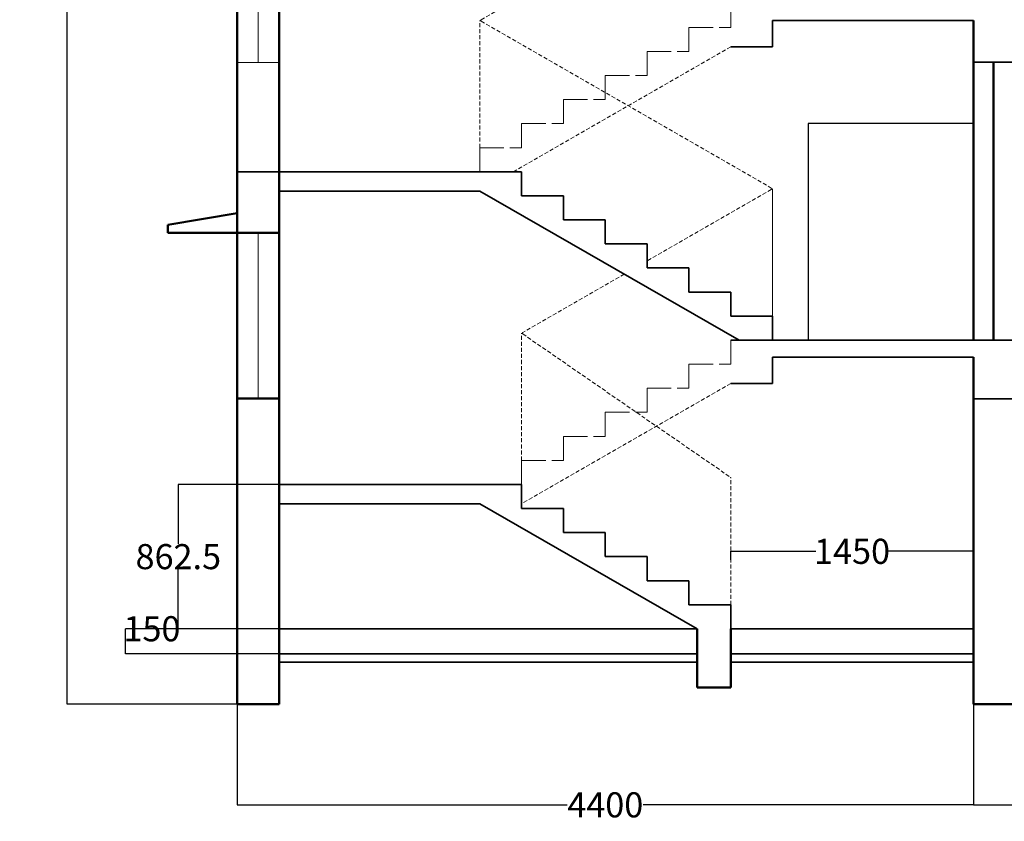
# Model space of a CAD drawing. Units: millimetres. Extents: x -1193 to 12449, y -949 to 12489.
# Tile 1 of 2: x -1193 to 4692, y -949 to 3842. Entities that reach past the tile are written whole.
import ezdxf

# ---------------------------------------------------------------- set-up
doc = ezdxf.new("R2010")
doc.units = ezdxf.units.MM
doc.header["$LTSCALE"] = 12
doc.header["$MEASUREMENT"] = 0
doc.linetypes.add('ACAD_ISO02W100', pattern=[15, 12, -3])
doc.linetypes.add('HIDDEN', pattern=[0.375, 0.25, -0.125])
for name, color, linetype, lineweight in [('A-ANNO-DIMS', 2, 'Continuous', 18), ('A-DOOR', 3, 'Continuous', 25), ('A-FLOR', 7, 'Continuous', 35), ('A-FLOR-HRAL-BYND', 8, 'ACAD_ISO02W100', 18), ('A-FLOR-HRAL-HIDN', 8, 'HIDDEN', 18), ('A-FLOR-STRS', 7, 'Continuous', 35), ('A-FLOR-STRS-BYND', 8, 'ACAD_ISO02W100', 18), ('A-FLOR-STRS-HIDN', 8, 'HIDDEN', 18), ('A-GLAZ', 4, 'Continuous', 18), ('A-WALL', 7, 'Continuous', 50), ('A-WALL-BYND', 8, 'ACAD_ISO02W100', 18), ('S-BEAM', 1, 'Continuous', 35), ('S-COLS', 1, 'Continuous', 50), ('S-FNDN', 1, 'Continuous', 50)]:
    doc.layers.add(name, color=color, linetype=linetype, lineweight=lineweight)
doc.styles.get("Standard").update_dxf_attribs({"font": 'arial.ttf'})
doc.dimstyles.get("Standard").update_dxf_attribs({"dimtxt": 150, "dimasz": 0.18, "dimexe": 0.18, "dimexo": 0.0625, "dimgap": 0.09, "dimtad": 0, "dimtih": 1, "dimtoh": 1, "dimdec": 0, "dimzin": 0, "dimdsep": 46, "dimtxsty": 'Standard', "dimcen": 0.09, "dimadec": 0, "dimazin": 0, "dimtfac": 1, "dimtdec": 0, "dimtofl": 0, "dimtmove": 0, "dimatfit": 3, "dimfxl": 1, "dimtolj": 1, "dimtzin": 0, "dimarcsym": 0})

# ---------------------------------------------------------------- blocks, each defined once
blk = doc.blocks.new('*D3')
at = {"layer": 'A-ANNO-DIMS', "color": 0, "lineweight": -2, "ltscale": 8, "transparency": 16777216}
for p, q in [((3057.011297115449, 613.4543490366777), (3057.011297115449, 664.80195058669)), ((3057.191297115449, 664.6219505866902), (3565.260314850783, 664.6219505866902)), ((4506.831297115448, 664.6219505866902), (3998.762279380115, 664.6219505866902)), ((4507.011297115449, 613.4543490366777), (4507.011297115449, 664.80195058669))]:
    blk.add_line(p, q, dxfattribs=at)
at = {"layer": 'A-ANNO-DIMS', "color": 0, "ltscale": 8, "transparency": 16777216}
for points in [[(3057.191297115449, 664.6519505866901), (3057.191297115449, 664.5919505866902), (3057.011297115449, 664.6219505866902)], [(4506.831297115448, 664.6519505866901), (4506.831297115448, 664.5919505866902), (4507.011297115449, 664.6219505866902)]]:
    blk.add_solid(points, dxfattribs=at)
at = {"layer": 'Defpoints', "color": 0, "ltscale": 8, "transparency": 16777216}
for p in [(4507.011297115449, 664.6219505866902), (3057.011297115449, 613.3918490366777), (4507.011297115449, 613.3918490366777)]:
    blk.add_point(p, dxfattribs=at)
at = {"layer": 'A-ANNO-DIMS', "color": 0, "ltscale": 8, "transparency": 16777216, "insert": (3782.011297115449, 664.6219505866902), "char_height": 150, "attachment_point": 5}
blk.add_mtext('\\A1;1450', dxfattribs=at)
blk = doc.blocks.new('*D5')
at = {"layer": 'A-ANNO-DIMS', "color": 0, "lineweight": -2, "ltscale": 8, "transparency": 16777216}
for p, q in [((356.9487971154486, 201.7493925244232), (-561.4085524250191, 201.749392524423)), ((-561.2285524250191, 201.749392524423), (-561.2285524250191, 201.929392524423)), ((-561.2285524250191, 201.929392524423), (-561.0485524250192, 201.929392524423)), ((-561.2285524250191, 51.92939252442293), (-561.2285524250191, 201.569392524423)), ((356.9487971154487, 51.74939252442309), (-561.4085524250191, 51.74939252442293))]:
    blk.add_line(p, q, dxfattribs=at)
at = {"layer": 'A-ANNO-DIMS', "color": 0, "ltscale": 8, "transparency": 16777216}
for points in [[(-561.258552425019, 201.569392524423), (-561.1985524250192, 201.569392524423), (-561.2285524250191, 201.749392524423)], [(-561.258552425019, 51.92939252442293), (-561.1985524250192, 51.92939252442293), (-561.2285524250191, 51.74939252442293)]]:
    blk.add_solid(points, dxfattribs=at)
at = {"layer": 'Defpoints', "color": 0, "ltscale": 8, "transparency": 16777216}
for p in [(-561.2285524250191, 201.749392524423), (357.0112971154486, 201.7493925244232), (357.0112971154487, 51.74939252442309)]:
    blk.add_point(p, dxfattribs=at)
at = {"layer": 'A-ANNO-DIMS', "color": 0, "ltscale": 8, "transparency": 16777216, "insert": (-402.5683750716766, 201.9293925244231), "char_height": 150, "attachment_point": 5}
blk.add_mtext('\\A1;150', dxfattribs=at)
blk = doc.blocks.new('STAIR-FLIGHT-LANDING-TYP')
at = {"ltscale": 8}
for p, q in [((1200, 1006.25), (-5.68e-14, 1006.25)), ((1200, 890.8972800494066), (-5.68e-14, 890.8972800494066))]:
    blk.add_line(p, q, dxfattribs=at)
for p, q in [((1450, 1006.25), (1200, 1006.25)), ((1450, 862.5), (1450, 1006.25)), ((1700, 862.5), (1450, 862.5)), ((1700, 718.75), (1700, 862.5)), ((1950, 718.75), (1700, 718.75)), ((1950, 575), (1950, 718.75)), ((2200, 575), (1950, 575)), ((2200, 431.25), (2200, 575)), ((2450, 431.25), (2200, 431.25)), ((2450, 287.5), (2450, 431.25)), ((2700, 287.5), (2450, 287.5)), ((2700, 143.75), (2700, 287.5)), ((2950, 143.75), (2700, 143.75)), ((2950, 0), (2950, 143.75))]:
    blk.add_line(p, q)
blk.add_lwpolyline([(1200, 890.8972800494066), (2749.386573998968, 0)], dxfattribs=at)
blk = doc.blocks.new('STAIR-RETURN-TYP')
for p, q in [((1500, 862.5), (1500, 1006.25)), ((1500, 1006.25), (1750, 1006.25)), ((1250, 718.75), (1250, 862.5)), ((1250, 862.5), (1500, 862.5)), ((999.9999999999995, 575), (999.9999999999995, 718.75)), ((999.9999999999995, 718.75), (1250, 718.75)), ((749.9999999999995, 431.25), (749.9999999999995, 575)), ((749.9999999999995, 575), (999.9999999999995, 575)), ((499.9999999999995, 287.5), (499.9999999999995, 431.25)), ((499.9999999999995, 431.25), (749.9999999999995, 431.25)), ((249.9999999999996, 143.75), (249.9999999999996, 287.5)), ((249.9999999999996, 287.5), (499.9999999999995, 287.5)), ((-4.547e-13, 0), (-4.547e-13, 143.75)), ((-4.547e-13, 143.75), (249.9999999999996, 143.75))]:
    blk.add_line(p, q)
blk = doc.blocks.new('DOOR-STAIR-OPENING')
at = {"ltscale": 8}
for p, q in [((988.0075403151895, 1293.961950984857), (0, 1293.961950984857)), ((0, 1293.961950984857), (0, 0))]:
    blk.add_line(p, q, dxfattribs=at)
blk = doc.blocks.new('BEAM-DROP-250x250')
for p, q in [((0, 250), (0, 0)), ((250, 0), (250, 250)), ((0, 0), (250, 0))]:
    blk.add_line(p, q)
blk = doc.blocks.new('*D28')
at = {"layer": 'A-ANNO-DIMS', "color": 0, "lineweight": -2, "ltscale": 8, "transparency": 16777216}
for p, q in [((106.948797, 11788.48548), (-909.1941130000021, 11788.48548)), ((-909.0141130000022, 11788.30548), (-909.0141130000007, 5846.844544276263)), ((-909.0141129999995, -248.0706070000003), (-909.0141130000007, 5693.39032872374)), ((106.948797, -248.2506070000001), (-909.1941129999994, -248.2506070000003))]:
    blk.add_line(p, q, dxfattribs=at)
at = {"layer": 'A-ANNO-DIMS', "color": 0, "ltscale": 8, "transparency": 16777216}
for points in [[(-909.0441130000021, 11788.30548), (-908.9841130000023, 11788.30548), (-909.0141130000022, 11788.48548)], [(-909.0441129999996, -248.0706070000003), (-908.9841129999996, -248.0706070000003), (-909.0141129999995, -248.2506070000003)]]:
    blk.add_solid(points, dxfattribs=at)
at = {"layer": 'Defpoints', "color": 0, "ltscale": 8, "transparency": 16777216}
for p in [(-909.0141130000022, 11788.48548), (107.011297, 11788.48548), (107.011297, -248.2506070000001)]:
    blk.add_point(p, dxfattribs=at)
at = {"layer": 'A-ANNO-DIMS', "color": 0, "ltscale": 8, "transparency": 16777216, "insert": (-909.014112999999, 5770.117436500001), "char_height": 150, "attachment_point": 5}
blk.add_mtext('\\A1;12037', dxfattribs=at)
blk = doc.blocks.new('*D29')
at = {"layer": 'A-ANNO-DIMS', "color": 0, "lineweight": -2, "ltscale": 8, "transparency": 16777216}
for p, q in [((107.011297, -248.313107), (107.0112969999999, -850.430607)), ((4507.011297, -248.313107), (4507.011297, -850.430607)), ((107.1912969999999, -850.250607), (2080.181869987722, -850.250607)), ((4506.831297, -850.250607), (2533.840724012279, -850.250607))]:
    blk.add_line(p, q, dxfattribs=at)
at = {"layer": 'A-ANNO-DIMS', "color": 0, "ltscale": 8, "transparency": 16777216}
for points in [[(107.1912969999999, -850.2206069999999), (107.1912969999999, -850.280607), (107.0112969999999, -850.250607)], [(4506.831297, -850.2206069999999), (4506.831297, -850.280607), (4507.011297, -850.250607)]]:
    blk.add_solid(points, dxfattribs=at)
at = {"layer": 'Defpoints', "color": 0, "ltscale": 8, "transparency": 16777216}
for p in [(107.011297, -248.250607), (4507.011297, -248.250607), (4507.011297, -850.250607)]:
    blk.add_point(p, dxfattribs=at)
at = {"layer": 'A-ANNO-DIMS', "color": 0, "ltscale": 8, "transparency": 16777216, "insert": (2307.011297, -850.250607), "char_height": 150, "attachment_point": 5}
blk.add_mtext('\\A1;4400', dxfattribs=at)
blk = doc.blocks.new('*D30')
at = {"layer": 'A-ANNO-DIMS', "color": 0, "lineweight": -2, "ltscale": 8, "transparency": 16777216}
for p, q in [((5559.096303, 2520.911284), (5559.096303, -850.4306069999998)), ((4507.011297, -248.313107), (4507.011297, -850.430607)), ((4507.191297000001, -850.250607), (4816.814413915416, -850.250607)), ((5558.916303, -850.250607), (5249.293186084583, -850.250607))]:
    blk.add_line(p, q, dxfattribs=at)
at = {"layer": 'A-ANNO-DIMS', "color": 0, "ltscale": 8, "transparency": 16777216}
for points in [[(4507.191297000001, -850.2206069999999), (4507.191297000001, -850.280607), (4507.011297, -850.250607)], [(5558.916303, -850.2206069999999), (5558.916303, -850.280607), (5559.096303, -850.250607)]]:
    blk.add_solid(points, dxfattribs=at)
at = {"layer": 'Defpoints', "color": 0, "ltscale": 8, "transparency": 16777216}
for p in [(5559.096303, 2520.973784), (4507.011297, -248.250607), (5559.096303, -850.250607)]:
    blk.add_point(p, dxfattribs=at)
at = {"layer": 'A-ANNO-DIMS', "color": 0, "ltscale": 8, "transparency": 16777216, "insert": (5033.0538, -850.250607), "char_height": 150, "attachment_point": 5}
blk.add_mtext('\\A1;1052', dxfattribs=at)
blk = doc.blocks.new('*D49')
at = {"layer": 'A-ANNO-DIMS', "color": 0, "lineweight": -2, "ltscale": 8, "transparency": 16777216}
for p, q in [((356.9487970000001, 1064.249393), (-245.1687030000003, 1064.249393)), ((-244.9887030000003, 1064.069393), (-244.9887030000002, 709.6753411582539)), ((-244.9887030000001, 201.929393), (-244.9887030000002, 556.3234448417464)), ((356.9487970000001, 201.7493930000001), (-245.168703, 201.749393))]:
    blk.add_line(p, q, dxfattribs=at)
at = {"layer": 'A-ANNO-DIMS', "color": 0, "ltscale": 8, "transparency": 16777216}
for points in [[(-245.0187030000003, 1064.069393), (-244.9587030000003, 1064.069393), (-244.9887030000003, 1064.249393)], [(-245.0187030000001, 201.929393), (-244.9587030000001, 201.929393), (-244.9887030000001, 201.749393)]]:
    blk.add_solid(points, dxfattribs=at)
at = {"layer": 'Defpoints', "color": 0, "ltscale": 8, "transparency": 16777216}
for p in [(-244.9887030000003, 1064.249393), (357.0112970000001, 1064.249393), (357.0112970000001, 201.7493930000001)]:
    blk.add_point(p, dxfattribs=at)
at = {"layer": 'A-ANNO-DIMS', "color": 0, "ltscale": 8, "transparency": 16777216, "insert": (-244.988703, 632.999393), "char_height": 150, "attachment_point": 5}
blk.add_mtext('\\A1;862.5', dxfattribs=at)

msp = doc.modelspace()

# ---------------------------------------------------------------- linework, layer by layer
at = {"layer": 'A-FLOR', "ltscale": 8}
for p, q in [((3307.011297115448, 3837.249392524423), (4507.011297115449, 3837.249392524423)), ((3057.011297115449, 1926.749392524423), (4507.011297115449, 1926.749392524423))]:
    msp.add_line(p, q, dxfattribs=at)
at = {"layer": 'A-FLOR'}
for p, q in [((4507.011297115449, 1926.749392524423), (10755.12605663696, 1926.749392524423)), ((3307.011297115448, 1825.149392524423), (4507.011297115449, 1825.149392524423)), ((357.0112971154486, 201.749392524423), (2856.397871114416, 201.749392524423)), ((3057.011297115449, 201.749392524423), (4507.011297115449, 201.749392524423)), ((357.0112971154486, 51.74939252442306), (2856.397871114416, 51.74939252442306)), ((357.0112971154486, 1.749392524423061), (2856.397871114416, 1.749392524423061)), ((3057.011297115448, 51.74939252442306), (4507.011297115449, 51.74939252442306)), ((3057.011297115448, 1.749392524423061), (4507.011297115449, 1.749392524423061))]:
    msp.add_line(p, q, dxfattribs=at)
at = {"layer": 'A-FLOR-HRAL-BYND', "ltscale": 8}
msp.add_line((3307.011297115449, 2070.499392524423), (3307.011297115449, 2830.999392524419), dxfattribs=at)
at = {"layer": 'A-FLOR-HRAL-HIDN', "ltscale": 8}
for p, q in [((1564.54961279421, 3841.583924039707), (2420.40023628885, 4333.698032549124)), ((1557.011297115449, 3076.749392524423), (1557.011297115449, 3837.249392524419)), ((1564.54961279421, 3832.914861009131), (3299.472981436688, 2835.333924039707)), ((3299.472981436688, 2826.664861009131), (2557.011297115449, 2399.749392524419)), ((2420.400236288849, 2321.198032549124), (1813.880505755374, 1972.449187492376)), ((1807.011297115449, 1207.999392524423), (1807.011297115449, 1968.499392524419)), ((1813.533234977974, 1963.999255399276), (3054.850923514139, 1107.490050309322)), ((3057.011297115449, 345.499392524423), (3057.011297115449, 1103.37464973151))]:
    msp.add_line(p, q, dxfattribs=at)
for centre, start, end in [((1567.0419684155, 3837.249392524419), 119.8989018386145, 240.1010981613854), ((3296.980625815397, 2830.999392524419), 299.8989018386146, 60.10109816138544), ((1816.372861376665, 1968.114655977089), 119.8989018386145, 235.3943244483614), ((3052.011297115449, 1103.37464973151), 0, 55.39432444836143)]:
    msp.add_arc(centre, 5, start, end, dxfattribs=at)
at = {"layer": 'A-FLOR-STRS', "ltscale": 8}
for p, q in [((3307.011297115449, 3679.746672573831), (3307.011297115448, 3837.249392524423)), ((3057.011297115449, 3679.746672573831), (3307.011297115449, 3679.746672573831)), ((357.0112971154486, 2932.999392524423), (107.0112971154485, 2932.999392524423)), ((3307.011297115449, 1667.64667257383), (3307.011297115448, 1825.149392524423)), ((3057.011297115449, 1667.64667257383), (3307.011297115449, 1667.64667257383))]:
    msp.add_line(p, q, dxfattribs=at)
at = {"layer": 'A-FLOR-STRS'}
for p, q in [((1557.011297115449, 1064.249392524423), (357.0112971154486, 1064.249392524423)), ((1807.011297115449, 1064.249392524423), (1557.011297115449, 1064.249392524423)), ((1807.011297115449, 920.4993925244229), (1807.011297115449, 1064.249392524423)), ((1557.011297115449, 948.8966725738297), (357.0112971154486, 948.8966725738297)), ((2057.011297115449, 920.4993925244229), (1807.011297115449, 920.4993925244229)), ((2057.011297115449, 776.749392524423), (2057.011297115449, 920.4993925244229)), ((2307.011297115449, 776.749392524423), (2057.011297115449, 776.749392524423)), ((2307.011297115449, 632.999392524423), (2307.011297115449, 776.749392524423)), ((2557.011297115449, 632.999392524423), (2307.011297115449, 632.999392524423)), ((2557.011297115449, 489.249392524423), (2557.011297115449, 632.999392524423)), ((2807.011297115449, 489.249392524423), (2557.011297115449, 489.249392524423)), ((2807.011297115449, 345.499392524423), (2807.011297115449, 489.249392524423)), ((3057.011297115449, 345.499392524423), (2807.011297115449, 345.499392524423)), ((3057.011297115449, 201.749392524423), (3057.011297115449, 345.499392524423))]:
    msp.add_line(p, q, dxfattribs=at)
msp.add_lwpolyline([(1557.011297115449, 948.8966725738297), (2856.397871114416, 201.7493925244232)], dxfattribs=at)
at = {"layer": 'A-FLOR-STRS-BYND'}
for p, q in [((3057.011297115449, 1782.999392524423), (3057.011297115449, 1926.749392524423)), ((2807.011297115449, 1639.249392524423), (2807.011297115449, 1782.999392524423)), ((2807.011297115449, 1782.999392524423), (3057.011297115449, 1782.999392524423)), ((2557.011297115449, 1495.499392524423), (2557.011297115449, 1639.249392524423)), ((2557.011297115449, 1639.249392524423), (2807.011297115449, 1639.249392524423)), ((2307.011297115449, 1351.749392524423), (2307.011297115449, 1495.499392524423)), ((2307.011297115449, 1495.499392524423), (2557.011297115449, 1495.499392524423)), ((2057.011297115449, 1207.999392524423), (2057.011297115449, 1351.749392524423)), ((2057.011297115449, 1351.749392524423), (2307.011297115449, 1351.749392524423)), ((1807.011297115449, 1064.249392524423), (1807.011297115449, 1207.999392524423)), ((1807.011297115449, 1207.999392524423), (2057.011297115449, 1207.999392524423))]:
    msp.add_line(p, q, dxfattribs=at)
at = {"layer": 'A-FLOR-STRS-HIDN', "ltscale": 8}
for points in [[(3057.011297115449, 3680.14667257383), (1757.62472311648, 2932.999392524423)], [(3057.011297115449, 1667.64667257383), (1807.011297115449, 948.8966725738298)]]:
    msp.add_lwpolyline(points, dxfattribs=at)
at = {"layer": 'A-GLAZ', "ltscale": 8}
for p, q in [((232.0112971154486, 3585.559064102367), (232.0112971154486, 4580.14667257383)), ((232.0112971154486, 1577.917477170344), (232.0112971154486, 2567.64667257383))]:
    msp.add_line(p, q, dxfattribs=at)
at = {"layer": 'A-WALL'}
for p, q in [((357.0112971154486, 1.749392524423001), (357.0112971154486, 6957.999392524424)), ((107.0112971154485, 1.749392524423001), (107.0112971154486, 6710.235030402279))]:
    msp.add_line(p, q, dxfattribs=at)
at = {"layer": 'A-WALL', "ltscale": 8}
for p, q in [((4507.011297115449, 1926.749392524423), (4507.011297115449, 3837.249392524423)), ((4627.011297115449, 1926.749392524423), (4627.011297115449, 3587.249392524423)), ((357.0112971154486, 2817.64667257383), (357.0112971154486, 2567.64667257383)), ((-307.0141126089075, 2616.497394422149), (107.0112971154485, 2685.23503040228)), ((-307.0141126089075, 2567.64667257383), (-307.0141126089075, 2616.497394422149)), ((107.0112971154485, 2567.64667257383), (-307.0141126089075, 2567.64667257383)), ((357.0112971154486, 2567.64667257383), (107.0112971154485, 2567.64667257383)), ((357.0112971154486, 1577.917477170344), (107.0112971154485, 1577.917477170344))]:
    msp.add_line(p, q, dxfattribs=at)
at = {"layer": 'A-WALL-BYND', "ltscale": 8}
msp.add_line((357.0112971154487, 3585.559064102367), (107.0112971154485, 3585.559064102367), dxfattribs=at)
at = {"layer": 'S-COLS'}
msp.add_line((4507.011297115449, 201.749392524423), (4507.011297115449, 1825.149392524423), dxfattribs=at)
at = {"layer": 'S-FNDN'}
for p, q in [((2856.397871114416, -148.2506074755769), (2856.397871114416, 201.749392524423)), ((3057.011297115449, 201.749392524423), (3057.011297115449, 1.749392524423061)), ((4507.011297115449, 1.749392524423061), (4507.011297115449, 201.749392524423)), ((107.0112971154485, -248.2506074755769), (107.0112971154485, 1.749392524423001)), ((357.0112971154486, 1.749392524423061), (357.0112971154486, -248.2506074755769)), ((3057.011297115449, 1.749392524423061), (3057.011297115449, -148.2506074755769)), ((4507.011297115449, -248.2506074755769), (4507.011297115449, 1.749392524423061)), ((3057.011297115449, -148.2506074755769), (2856.397871114416, -148.2506074755769)), ((357.0112971154486, -248.2506074755769), (107.0112971154485, -248.2506074755769)), ((4757.011297115449, -248.2506074755769), (4507.011297115449, -248.2506074755769))]:
    msp.add_line(p, q, dxfattribs=at)

# ---------------------------------------------------------------- block references
at = {"layer": 'A-DOOR'}
msp.add_blockref('DOOR-STAIR-OPENING', (3519.003756800259, 1926.749392524423), dxfattribs=at)
at = {"layer": 'A-FLOR-STRS'}
msp.add_blockref('STAIR-FLIGHT-LANDING-TYP', (357.0112971154486, 1926.749392524423), dxfattribs=at)
at = {"layer": 'A-FLOR-STRS-BYND'}
msp.add_blockref('STAIR-RETURN-TYP', (1557.011297115449, 2932.999392524423), dxfattribs=at)
at = {"layer": 'S-BEAM'}
for p in [(4507.011297115449, 3587.249392524423), (4507.011297115449, 1575.149392524423)]:
    msp.add_blockref('BEAM-DROP-250x250', p, dxfattribs=at)

# ---------------------------------------------------------------- dimensions: what is measured, and where the dimension line sits
at = {"layer": 'A-ANNO-DIMS', "ltscale": 8}
for base, p1, p2, override, picture, middle in [((-909.0141130000022, 11788.48548), (107.011297, -248.250607), (107.011297, 11788.48548), {"dimdec": 0, "dimlfac": 1, "dimrnd": 0, "dimzin": 0, "dimdsep": 46, "dimlunit": 2}, '*D28', (-909.014112999999, 5770.117436500001)), ((-244.9887030000003, 1064.249393), (357.011297, 201.749393), (357.011297, 1064.249393), {"dimdec": 1, "dimlfac": 1, "dimrnd": 0, "dimzin": 0, "dimdsep": 46, "dimlunit": 2}, '*D49', (-244.988703, 632.999393))]:
    dim = msp.add_linear_dim(base=base, p1=p1, p2=p2, angle=90, dimstyle='Standard', override=override, dxfattribs=at)
    dim.commit()
    dim.dimension.update_dxf_attribs({"geometry": picture, "text_midpoint": middle})
for base, p1, p2, picture, middle in [((5559.096303, -850.250607), (4507.011297, -248.250607), (5559.096303, 2520.973784), '*D30', (5033.0538, -850.250607)), ((4507.011297, -850.250607), (107.011297, -248.250607), (4507.011297, -248.250607), '*D29', (2307.011297, -850.250607))]:
    dim = msp.add_linear_dim(base=base, p1=p1, p2=p2, dimstyle='Standard', override={"dimdec": 0, "dimlfac": 1, "dimrnd": 0, "dimzin": 0, "dimdsep": 46, "dimlunit": 2}, dxfattribs=at)
    dim.commit()
    dim.dimension.update_dxf_attribs({"geometry": picture, "text_midpoint": middle})
for p1, p2, distance, picture, middle in [((3057.011297115449, 613.3918490366777), (4507.011297115449, 613.3918490366777), 51.230101550012485, '*D3', (3782.011297115449, 664.6219505866902)), ((357.0112971154486, 51.74939252442306), (357.0112971154485, 201.749392524423), 918.2398495404676, '*D5', (-402.5683750716766, 201.9293925244231))]:
    dim = msp.add_aligned_dim(p1=p1, p2=p2, distance=distance, dimstyle='Standard', override={"dimclrd": 0, "dimclre": 0, "dimclrt": 0}, dxfattribs=at)
    dim.commit()
    dim.dimension.update_dxf_attribs({"geometry": picture, "text_midpoint": middle})

doc.saveas('drawing.dxf')
